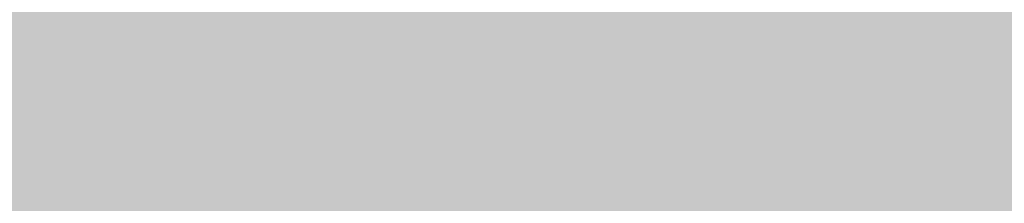
# Model space of a CAD drawing. Units: feet. Extents: x 3168 to 4724, y 827 to 1477.
# Tile 29 of 256: x 3261.901 to 3270.273, y 1096.781 to 1098.344. Entities that reach past the tile are written whole.
import ezdxf

# ---------------------------------------------------------------- set-up
doc = ezdxf.new("R2010")
doc.units = ezdxf.units.FT
doc.layers.add('A-ELEV-PATT', color=8, linetype='Continuous', lineweight=13)

msp = doc.modelspace()

# ---------------------------------------------------------------- hatches: boundary and pattern name
at = {"layer": 'A-ELEV-PATT'}
h = msp.add_hatch(color=256, dxfattribs=at)
h.dxf.hatch_style = 1
edge = h.paths.add_edge_path()
edge.add_ellipse((3552.9058, 979.2201), major_axis=(36.7449, 0), ratio=0.4848485, start_angle=0, end_angle=360)
edge = h.paths.add_edge_path()
edge.add_ellipse((3559.8916, 929.2523), major_axis=(36.7449, 0), ratio=0.4848485, start_angle=0, end_angle=360)
edge = h.paths.add_edge_path()
edge.add_line((3299.3168, 1198.6061), (3479.9167, 1198.6061))
edge.add_line((3479.9167, 1198.6061), (3479.9167, 1209.8686))
edge.add_spline(control_points=[(3479.9167, 1209.8686), (3464.3012, 1209.8686), (3448.6856, 1209.8686), (3410.9491, 1209.8686), (3388.8282, 1209.8686), (3355.6469, 1209.8686), (3344.5864, 1209.8686), (3327.9957, 1209.8686), (3322.4655, 1209.8686), (3314.1702, 1209.8686), (3311.4051, 1209.8686), (3307.2574, 1209.8686), (3305.8748, 1209.8686), (3303.801, 1209.8686), (3303.1097, 1209.8686), (3302.0728, 1209.8686), (3301.7272, 1209.8686), (3301.2087, 1209.8686), (3301.0359, 1209.8686), (3300.7767, 1209.8686), (3300.6903, 1209.8686), (3300.5606, 1209.8686), (3300.5174, 1209.8686), (3300.4526, 1209.8686), (3300.431, 1209.8686), (3300.3986, 1209.8686), (3300.3878, 1209.8686), (3300.3662, 1209.8686), (3300.3457, 1209.8686), (3300.3455, 1209.8686), (3300.3455, 1209.8686), (3300.3433, 1209.8686), (3300.3411, 1209.8686), (3300.3379, 1209.8686), (3300.3368, 1209.8686), (3300.3339, 1209.8686), (3300.3321, 1209.8686), (3300.3255, 1209.8686), (3300.3207, 1209.8686), (3300.3109, 1209.8686), (3300.306, 1209.8686), (3300.2905, 1209.8686), (3300.28, 1209.8686), (3300.2324, 1209.8688), (3300.1953, 1209.869), (3299.9511, 1209.8706), (3299.7448, 1209.8743), (3299.4368, 1209.8833), (3299.3344, 1209.8868), (3299.1811, 1209.8929), (3299.13, 1209.8951), (3298.6522, 1209.9168), (3298.2295, 1209.9457), (3297.6016, 1210.0024), (3297.3934, 1210.0235), (3297.0827, 1210.0583), (3296.9793, 1210.0705), (3296.293, 1210.1549), (3295.7181, 1210.2434), (3294.8687, 1210.3989), (3294.5877, 1210.4545), (3294.1693, 1210.5433), (3294.0304, 1210.5739), (3291.7071, 1211.1012), (3289.6536, 1211.8134), (3285.7763, 1213.564), (3283.9514, 1214.6035), (3280.5122, 1216.9801), (3278.8972, 1218.3176), (3276.3799, 1220.8295), (3275.416, 1221.9177), (3274.0393, 1223.7077), (3273.581, 1224.3495), (3273.1432, 1225.0163)], knot_values=[39.119033, 39.119033, 39.119033, 39.119033, 39.286353, 39.286353, 39.523379, 39.523379, 39.641892, 39.641892, 39.701148, 39.701148, 39.730777, 39.730777, 39.745591, 39.745591, 39.752998, 39.752998, 39.756701, 39.756701, 39.758553, 39.758553, 39.759479, 39.759479, 39.759942, 39.759942, 39.760173, 39.760173, 39.760289, 39.760289, 39.760405, 39.760405, 39.760463, 39.760463, 39.763389, 39.763389, 39.764851, 39.764851, 39.767304, 39.767304, 39.773825, 39.773825, 39.78057, 39.78057, 39.79477, 39.79477, 39.845194, 39.845194, 40.126715, 40.126715, 40.267476, 40.267476, 40.337856, 40.337856, 40.927023, 40.927023, 41.221606, 41.221606, 41.368898, 41.368898, 42.202622, 42.202622, 42.619485, 42.619485, 42.827916, 42.827916, 46.118323, 46.118323, 49.408731, 49.408731, 52.699139, 52.699139, 54.927489, 54.927489, 56.104228, 56.104228, 56.104228, 56.104228], weights=[1, 1, 1, 1, 1, 1, 1, 1, 1, 1, 1, 1, 1, 1, 1, 1, 1, 1, 1, 1, 1, 1, 1, 1, 1, 1, 1, 1, 1, 1, 1, 1, 1, 1, 1, 1, 1, 1, 1, 1, 1, 1, 1, 1, 1, 1, 1, 1, 1, 1, 1, 1, 1, 1, 1, 1, 1, 1, 1, 1, 1, 1, 1, 1, 1, 1, 1, 1, 1, 1, 1, 1, 1, 1], degree=3, periodic=0)
edge.add_line((3273.1432, 1225.0163), (3273.1432, 1099.0163))
edge.add_line((3273.1432, 1099.0163), (3299.3168, 1099.0163))
edge.add_line((3299.3168, 1099.0163), (3299.3168, 1198.6061))
edge = h.paths.add_edge_path()
edge.add_line((3304.7584, 1324.1581), (3479.9167, 1324.1581))
edge.add_line((3479.9167, 1324.1581), (3479.9167, 1335.7146))
edge.add_line((3479.9167, 1335.7146), (3269.1616, 1335.7146))
edge.add_spline(control_points=[(3269.1616, 1335.7146), (3264.0242, 1335.7146), (3258.3641, 1328.9582), (3259.2643, 1323.9003)], knot_values=[0, 0, 0, 0, 15.412191, 15.412191, 15.412191, 15.412191], degree=3, periodic=0)
edge.add_line((3259.2643, 1323.9003), (3265.5168, 1288.7691))
edge.add_line((3265.5168, 1288.7691), (3275.2651, 1261.5456))
edge.add_line((3275.2651, 1261.5456), (3304.7584, 1261.5456))
edge.add_line((3304.7584, 1261.5456), (3304.7584, 1324.1581))
h = msp.add_hatch(color=256, dxfattribs=at)
h.dxf.hatch_style = 1
h.paths.add_polyline_path([(3384.5252, 1099.0163), (3335.0292, 1099.0163), (3299.3168, 1099.0163), (3273.1432, 1099.0163), (3217.5654, 1099.0163), (3168.0693, 827.1163), (3335.0292, 827.1163)])

doc.saveas('drawing.dxf')
